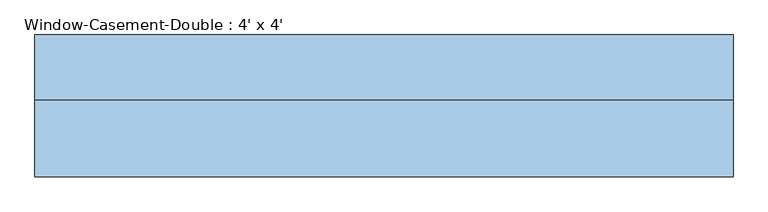
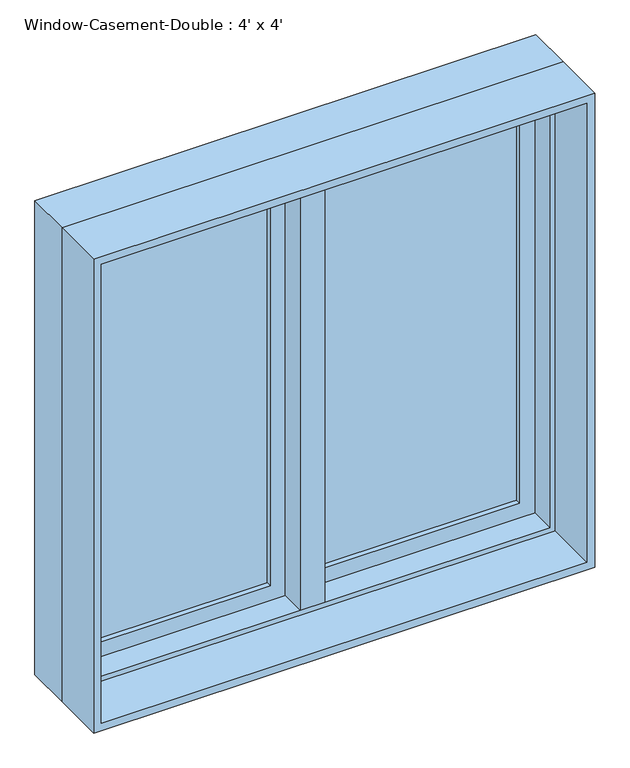
"""IFC4 building model written with IfcOpenShell, lengths in millimetres: window geometry, Window-Casement-Double : 4' x 4'."""

from ifc_helpers import new_model, si_unit, frame, origin, place, context, project, spatial, polyline, outline, extrude, faceted_brep, source, transform, mapped, element, save


def window_casement_double_4_x_4_af3140d2(model_context):
    return source(origin(), model_context, "Body", "SolidModel", [
        faceted_brep([(9.525, 133.35, 2120.9), (-9.525, 133.35, 2120.9), (-9.525, 82.55, 2120.9), (9.525, 82.55, 2120.9), (9.525, 133.35, 927.1), (9.525, 82.55, 927.1), (-9.525, 82.55, 927.1), (-9.525, 133.35, 927.1), (-9.525, 82.55, 946.15), (-9.525, 82.55, 2101.85), (-30.1625, 82.55, 946.15), (-30.1625, 82.55, 2101.85), (-30.1625, 19.05, 946.15), (-30.1625, 19.05, 2101.85), (30.1625, 19.05, 946.15), (30.1625, 19.05, 2101.85), (30.1625, 82.55, 946.15), (30.1625, 82.55, 2101.85), (9.525, 82.55, 946.15), (9.525, 82.55, 2101.85)], [[[0, 1, 2, 3]], [[4, 5, 6, 7]], [[1, 0, 4, 7]], [[2, 1, 7, 6, 8, 9]], [[9, 8, 10, 11]], [[11, 10, 12, 13]], [[13, 12, 14, 15]], [[15, 14, 16, 17]], [[17, 16, 18, 19]], [[0, 3, 19, 18, 5, 4]], [[18, 8, 6, 5]], [[9, 19, 3, 2]], [[8, 18, 16, 14, 12, 10]], [[19, 9, 11, 13, 15, 17]]]),
        extrude(outline(polyline([(-66.675, 114.3), (-66.675, 107.95), (-539.75, 107.95), (-539.75, 114.3), (-66.675, 114.3)])), frame((0.0, 0.0, 984.25), z_axis=(0.0, 0.0, 1.0), x_axis=(1.0, 0.0, 0.0)), (0.0, 0.0, 1.0), 1079.5),
        extrude(outline(polyline([(-539.75, 95.25), (-539.75, 101.6), (-66.675, 101.6), (-66.675, 95.25), (-539.75, 95.25)])), frame((0.0, 0.0, 984.25), z_axis=(0.0, 0.0, 1.0), x_axis=(1.0, 0.0, 0.0)), (0.0, 0.0, 1.0), 1079.5),
        extrude(outline(polyline([(539.75, 114.3), (539.75, 107.95), (66.675, 107.95), (66.675, 114.3), (539.75, 114.3)])), frame((0.0, 0.0, 984.25), z_axis=(0.0, 0.0, 1.0), x_axis=(1.0, 0.0, 0.0)), (0.0, 0.0, 1.0), 1079.5),
        extrude(outline(polyline([(66.675, 95.25), (66.675, 101.6), (539.75, 101.6), (539.75, 95.25), (66.675, 95.25)])), frame((0.0, 0.0, 984.25), z_axis=(0.0, 0.0, 1.0), x_axis=(1.0, 0.0, 0.0)), (0.0, 0.0, 1.0), 1079.5),
        extrude(outline(polyline([(2120.9, -596.9), (927.1, -596.9), (927.1, -9.525), (2120.9, -9.525), (2120.9, -596.9)]), holes=[polyline([(2063.75, -66.675), (984.25, -66.675), (984.25, -539.75), (2063.75, -539.75), (2063.75, -66.675)])]), frame((0.0, 82.55, 0.0), z_axis=(0.0, 1.0, 0.0), x_axis=(0.0, 0.0, 1.0)), (0.0, 0.0, 1.0), 44.45),
        extrude(outline(polyline([(927.1, 596.9), (2120.9, 596.9), (2120.9, 9.525), (927.1, 9.525), (927.1, 596.9)]), holes=[polyline([(984.25, 66.675), (2063.75, 66.675), (2063.75, 539.75), (984.25, 539.75), (984.25, 66.675)])]), frame((0.0, 82.55, 0.0), z_axis=(0.0, 1.0, 0.0), x_axis=(0.0, 0.0, 1.0)), (0.0, 0.0, 1.0), 44.45),
        extrude(outline(polyline([(2133.6, -609.6), (914.4, -609.6), (914.4, 609.6), (2133.6, 609.6), (2133.6, -609.6)]), holes=[polyline([(2114.55, 590.55), (933.45, 590.55), (933.45, -590.55), (2114.55, -590.55), (2114.55, 590.55)])]), frame((0.0, -114.3, 0.0), z_axis=(0.0, 1.0, 0.0), x_axis=(0.0, 0.0, 1.0)), (0.0, 0.0, 1.0), 133.35),
        faceted_brep([(577.85, 82.55, 2101.85), (577.85, 19.05, 2101.85), (-577.85, 19.05, 2101.85), (-577.85, 82.55, 2101.85), (596.9, 133.35, 2120.9), (596.9, 82.55, 2120.9), (-596.9, 82.55, 2120.9), (-596.9, 133.35, 2120.9), (609.6, 19.05, 2133.6), (609.6, 133.35, 2133.6), (-609.6, 133.35, 2133.6), (-609.6, 19.05, 2133.6), (-577.85, 19.05, 946.15), (-577.85, 82.55, 946.15), (-596.9, 82.55, 927.1), (-596.9, 133.35, 927.1), (-609.6, 133.35, 914.4), (-609.6, 19.05, 914.4), (577.85, 19.05, 946.15), (577.85, 82.55, 946.15), (596.9, 82.55, 927.1), (596.9, 133.35, 927.1), (609.6, 133.35, 914.4), (609.6, 19.05, 914.4)], [[[0, 1, 2, 3]], [[4, 5, 6, 7]], [[8, 9, 10, 11]], [[3, 2, 12, 13]], [[7, 6, 14, 15]], [[11, 10, 16, 17]], [[13, 12, 18, 19]], [[15, 14, 20, 21]], [[17, 16, 22, 23]], [[11, 17, 23, 8], [1, 18, 12, 2]], [[19, 18, 1, 0]], [[5, 20, 14, 6], [3, 13, 19, 0]], [[21, 20, 5, 4]], [[23, 22, 9, 8]], [[9, 22, 16, 10], [7, 15, 21, 4]]]),
    ])


if __name__ == "__main__":
    model = new_model("IFC4")
    model_context = context("Model", 3, world=origin())
    ifc_project = project(units=[si_unit("LENGTHUNIT", "METRE", prefix="MILLI")], contexts=[model_context])
    site = spatial("IfcSite", under=ifc_project)
    building = spatial("IfcBuilding", under=site)
    placement = place(None, origin())
    window_casement_double_4_x_4_shape = window_casement_double_4_x_4_af3140d2(model_context)
    element("IfcWindow", 1, ObjectType="Window-Casement-Double : 4' x 4'", at=placement, inside=building, context=model_context, shape_type="MappedRepresentation", body=[
        mapped(window_casement_double_4_x_4_shape, transform((0.0, 0.0, 0.0), x_axis=(1.0, 0.0, 0.0), y_axis=(0.0, 1.0, 0.0), z_axis=(0.0, 0.0, 1.0))),
    ])
    save(model, "model.ifc")

# Revit data of these elements
# Type "Window-Casement-Double : 4' x 4'"
#   Type Mark = "21"
#   Fire Rating = "0.5h"
#   Assembly Code = "B2020100"
#   Analytic Construction = "Double glazing - domestic"
#   Frame Extension [instance default] = 0' - 0 1/4"
#   Window Inset [instance default] = 0' - 0"
#   Wall Thickness [instance default] = 0' - 6"
#   Interior Wall Closure [instance default] = 0' - 2 1/4"
#   Half Width = 2' - 0"
#   Visual Light Transmittance = 0.81
#   Thermal Resistance (R) = 1.8146 (h·ft²·°F)/BTU
#   Solar Heat Gain Coefficient = 0.76
#   Rough Width = 4' - 0 1/2"
#   Rough Height = 4' - 0 1/2"
#   Height = 4' - 0"
#   Heat Transfer Coefficient (U) = 0.5511 BTU/(h·ft²·°F)
#   Exterior Wall Closure [instance default] = 0' - 1 1/4"
#   Extension Jamb [instance default] = 0' - 2 1/4"
#   Default Sill Height = 3' - 0"
#   Width = 4' - 0"
#   Muntin Visibility = yes
#   Interior Trim Visibility [instance default] = yes
#   Exterior Trim Visibility [instance default] = yes
#   Extension Jamb Visibility [instance default] = yes
#   Interior Trim Material = Wood - Stained
#   Muntin Pattern = Muntin Pattern_2x2 : Muntin Pattern_2x2
#   Interior Trim = Trim-Window-Interior-Flat : Picture Frame
#   Interior Frame Material = Wood - Stained
#   Glass Panel Material = Glass
#   Exterior Trim Material = Clad - White
#   Exterior Trim = Trim-Window-Exterior-Flat : with Sill
#   Exterior Frame Material = Clad - White
#   Wall Closure = (empty or 0)
# Element 1 (IfcWindow, "Window-Casement-Double : 4' x 4'")
#   Wall Thickness = 0' - 9"
#   Extension Jamb = 0' - 5 1/4"
#   Materials on its faces: "Wood - Stained", "Glass", "Clad - White"
# Materials
#   "Wood - Stained": class "Wood", colour RGB 224 178 126, transparency 0, Cost = 0
#   "Glass": class "Glass", colour RGB 0 128 192, transparency 0.75, Description = "Soda Lime Glass", Cost = 0
#   "Clad - White": class "Wood", colour RGB 242 242 238, transparency 0, Cost = 0
